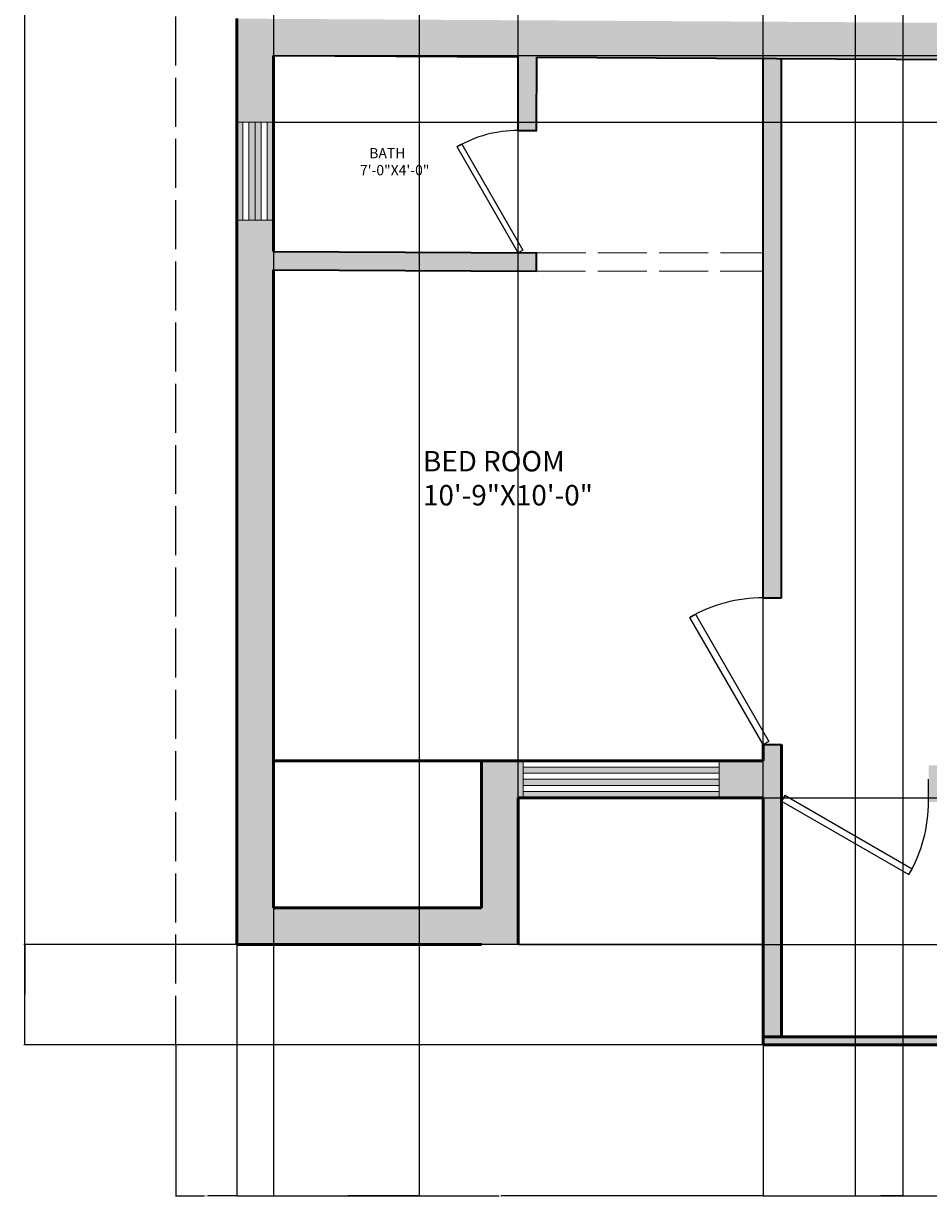
# Model space of a CAD drawing. Units: feet. Extents: x 2512 to 3087, y 1456 to 2266.
# Tile 1 of 5: x 2512 to 2734, y 1456 to 1744. Entities that reach past the tile are written whole.
import ezdxf

# ---------------------------------------------------------------- set-up
doc = ezdxf.new("R2010")
doc.units = ezdxf.units.FT
doc.linetypes.add('ACAD_ISO02W100', pattern=[15, 12, -3])
for name, color, linetype, lineweight in [('A-ANNO-DIMS', 2, 'Continuous', 18), ('A-DOOR', 240, 'Continuous', 25), ('A-GLAZ', 4, 'Continuous', 18), ('A-GLAZ-PATT', 252, 'Continuous', 13), ('A-WALL-OVHD', 8, 'ACAD_ISO02W100', 18), ('A-WALL-PATT', 252, 'Continuous', 13), ('ANNOTATION', 80, 'Continuous', 18), ('C-PROP', 8, 'ACAD_ISO02W100', 25), ('INNER WALL', 7, 'Continuous', 35), ('OPEN DOOR', 50, 'ACAD_ISO02W100', 18), ('OUTER WALL', 7, 'Continuous', 50)]:
    doc.layers.add(name, color=color, linetype=linetype, lineweight=lineweight)
doc.styles.get("Standard").update_dxf_attribs({"font": 'arial.ttf'})
doc.dimstyles.get("Standard").update_dxf_attribs({"dimtxt": 0.18, "dimasz": 0.18, "dimexe": 0.18, "dimexo": 0.0625, "dimgap": 0.09, "dimtad": 0, "dimtih": 1, "dimtoh": 1, "dimdec": 4, "dimzin": 0, "dimdsep": 46, "dimtxsty": 'Standard', "dimcen": 0.09, "dimadec": 0, "dimazin": 0, "dimtfac": 1, "dimtdec": 4, "dimtofl": 0, "dimtmove": 0, "dimatfit": 3, "dimfxl": 1, "dimtolj": 1, "dimtzin": 0, "dimarcsym": 0})

# ---------------------------------------------------------------- blocks, each defined once
blk = doc.blocks.new('*U8')
for p, q in [((0, 0), (0, 6)), ((40, 0), (40, 6))]:
    blk.add_line(p, q)
blk.add_lwpolyline([(0, 0), (34.64, -20), (35.52, -18.48), (0.87, 1.52)], close=True)
blk.add_arc((0, 0), 40, 330, 0)
blk = doc.blocks.new('*U9')
for p, q in [((-40, 0), (-40, 5)), ((0, 0), (0, 5))]:
    blk.add_line(p, q)
blk.add_lwpolyline([(0, 0), (-34.64, -20), (-35.52, -18.48), (-0.88, 1.52)], close=True)
blk.add_arc((0, 0), 40, 180, 210)
blk = doc.blocks.new('*U4')
for p, q in [((-40, 0), (-40, 6)), ((0, 0), (0, 6))]:
    blk.add_line(p, q)
blk.add_lwpolyline([(0, 0), (-34.64, -20), (-35.52, -18.48), (-0.87, 1.52)], close=True)
blk.add_arc((0, 0), 40, 180, 210)
blk = doc.blocks.new('VENT-24IN')
h = blk.add_hatch(color=256)
h.dxf.hatch_style = 1
h.paths.add_polyline_path([(24, 7.5), (24, 9), (0, 9), (0, 7.5)])
h.paths.add_polyline_path([(0, 1.5), (0, 0), (24, 0), (24, 1.5)])
h.paths.add_polyline_path([(0, 4.5), (0, 3), (24, 3), (24, 4.5)])
h.paths.add_polyline_path([(24, 4.5), (24, 6), (0, 6), (0, 4.5)])
for p, q in [((0, 9), (24, 9)), ((0, 0), (0, 9)), ((24, 9), (24, 0)), ((0, 7.5), (24, 7.5)), ((0, 6), (24, 6)), ((0, 4.5), (24, 4.5)), ((0, 3), (24, 3)), ((0, 1.5), (24, 1.5)), ((24, 0), (0, 0))]:
    blk.add_line(p, q)
blk = doc.blocks.new('*D18')
at = {"layer": 'A-ANNO-DIMS', "color": 0, "lineweight": -2, "transparency": 16777216}
for p, q in [((2549.23, 2229.02), (2512.11, 2229.02)), ((2512.29, 2228.84), (2512.29, 1861.31)), ((2512.29, 1493.41), (2512.29, 1860.94)), ((2549.23, 1493.23), (2512.11, 1493.23))]:
    blk.add_line(p, q, dxfattribs=at)
at = {"layer": 'A-ANNO-DIMS', "color": 0, "transparency": 16777216}
for points in [[(2512.26, 2228.84), (2512.32, 2228.84), (2512.29, 2229.02)], [(2512.26, 1493.41), (2512.32, 1493.41), (2512.29, 1493.23)]]:
    blk.add_solid(points, dxfattribs=at)
at = {"layer": 'Defpoints', "color": 0, "transparency": 16777216}
for p in [(2512.29, 2229.02), (2549.29, 2229.02), (2549.29, 1493.23)]:
    blk.add_point(p, dxfattribs=at)
at = {"layer": 'A-ANNO-DIMS', "color": 0, "transparency": 16777216, "insert": (2512.29, 1861.13), "char_height": 0.18, "attachment_point": 5}
blk.add_mtext('\\A1;735.8', dxfattribs=at)
blk = doc.blocks.new('*D20')
at = {"layer": 'A-ANNO-DIMS', "color": 0, "lineweight": -2, "transparency": 16777216}
for p, q in [((2564.16, 2213.23), (2512.11, 2213.23)), ((2512.29, 2213.05), (2512.29, 1853.41)), ((2512.29, 1493.41), (2512.29, 1853.05)), ((2693.16, 1493.23), (2512.11, 1493.23))]:
    blk.add_line(p, q, dxfattribs=at)
at = {"layer": 'A-ANNO-DIMS', "color": 0, "transparency": 16777216}
for points in [[(2512.26, 2213.05), (2512.32, 2213.05), (2512.29, 2213.23)], [(2512.26, 1493.41), (2512.32, 1493.41), (2512.29, 1493.23)]]:
    blk.add_solid(points, dxfattribs=at)
at = {"layer": 'Defpoints', "color": 0, "transparency": 16777216}
for p in [(2512.29, 2213.23), (2564.22, 2213.23), (2693.22, 1493.23)]:
    blk.add_point(p, dxfattribs=at)
at = {"layer": 'A-ANNO-DIMS', "color": 0, "transparency": 16777216, "insert": (2512.29, 1853.23), "char_height": 0.18, "attachment_point": 5}
blk.add_mtext('\\A1;720', dxfattribs=at)
blk = doc.blocks.new('*D21')
at = {"layer": 'A-ANNO-DIMS', "color": 0, "lineweight": -2, "transparency": 16777216}
for p, q in [((2573.22, 2204.17), (2573.22, 1456.05)), ((2608.89, 2204.17), (2608.89, 1456.05)), ((2573.4, 1456.23), (2590.66, 1456.23)), ((2608.71, 1456.23), (2591.45, 1456.23))]:
    blk.add_line(p, q, dxfattribs=at)
at = {"layer": 'A-ANNO-DIMS', "color": 0, "transparency": 16777216}
for points in [[(2573.4, 1456.26), (2573.4, 1456.2), (2573.22, 1456.23)], [(2608.71, 1456.26), (2608.71, 1456.2), (2608.89, 1456.23)]]:
    blk.add_solid(points, dxfattribs=at)
at = {"layer": 'Defpoints', "color": 0, "transparency": 16777216}
for p in [(2573.22, 2204.23), (2608.89, 2204.23), (2608.89, 1456.23)]:
    blk.add_point(p, dxfattribs=at)
at = {"layer": 'A-ANNO-DIMS', "color": 0, "transparency": 16777216, "insert": (2591.05, 1456.23), "char_height": 0.18, "attachment_point": 5}
blk.add_mtext('\\A1;35.67', dxfattribs=at)
blk = doc.blocks.new('*D22')
at = {"layer": 'A-ANNO-DIMS', "color": 0, "lineweight": -2, "transparency": 16777216}
for p, q in [((2715.72, 2204.17), (2715.72, 1456.05)), ((2727.45, 2204.17), (2727.45, 1456.05)), ((2715.9, 1456.23), (2721.13, 1456.23)), ((2727.27, 1456.23), (2722.04, 1456.23))]:
    blk.add_line(p, q, dxfattribs=at)
at = {"layer": 'A-ANNO-DIMS', "color": 0, "transparency": 16777216}
for points in [[(2715.9, 1456.26), (2715.9, 1456.2), (2715.72, 1456.23)], [(2727.27, 1456.26), (2727.27, 1456.2), (2727.45, 1456.23)]]:
    blk.add_solid(points, dxfattribs=at)
at = {"layer": 'Defpoints', "color": 0, "transparency": 16777216}
for p in [(2715.72, 2204.23), (2727.45, 2204.23), (2727.45, 1456.23)]:
    blk.add_point(p, dxfattribs=at)
at = {"layer": 'A-ANNO-DIMS', "color": 0, "transparency": 16777216, "insert": (2721.58, 1456.23), "char_height": 0.18, "attachment_point": 5}
blk.add_mtext('\\A1;11.729', dxfattribs=at)
blk = doc.blocks.new('*D25')
at = {"layer": 'A-ANNO-DIMS', "color": 0, "lineweight": -2, "transparency": 16777216}
for p, q in [((2564.22, 1517.74), (2564.22, 1456.05)), ((2549.29, 1493.17), (2549.29, 1456.05)), ((2549.47, 1456.23), (2556.37, 1456.23)), ((2564.04, 1456.23), (2557.14, 1456.23))]:
    blk.add_line(p, q, dxfattribs=at)
at = {"layer": 'A-ANNO-DIMS', "color": 0, "transparency": 16777216}
for points in [[(2549.47, 1456.26), (2549.47, 1456.2), (2549.29, 1456.23)], [(2564.04, 1456.26), (2564.04, 1456.2), (2564.22, 1456.23)]]:
    blk.add_solid(points, dxfattribs=at)
at = {"layer": 'Defpoints', "color": 0, "transparency": 16777216}
for p in [(2564.22, 1517.8), (2549.29, 1493.23), (2564.22, 1456.23)]:
    blk.add_point(p, dxfattribs=at)
at = {"layer": 'A-ANNO-DIMS', "color": 0, "transparency": 16777216, "insert": (2556.75, 1456.23), "char_height": 0.18, "attachment_point": 5}
blk.add_mtext('\\A1;14.93', dxfattribs=at)
blk = doc.blocks.new('*D26')
at = {"layer": 'A-ANNO-DIMS', "color": 0, "lineweight": -2, "transparency": 16777216}
for p, q in [((2564.22, 1517.74), (2564.22, 1456.05)), ((2693.22, 1493.17), (2693.22, 1456.05)), ((2564.4, 1456.23), (2628.44, 1456.23)), ((2693.04, 1456.23), (2629, 1456.23))]:
    blk.add_line(p, q, dxfattribs=at)
at = {"layer": 'A-ANNO-DIMS', "color": 0, "transparency": 16777216}
for points in [[(2564.4, 1456.26), (2564.4, 1456.2), (2564.22, 1456.23)], [(2693.04, 1456.26), (2693.04, 1456.2), (2693.22, 1456.23)]]:
    blk.add_solid(points, dxfattribs=at)
at = {"layer": 'Defpoints', "color": 0, "transparency": 16777216}
for p in [(2564.22, 1517.8), (2693.22, 1493.23), (2693.22, 1456.23)]:
    blk.add_point(p, dxfattribs=at)
at = {"layer": 'A-ANNO-DIMS', "color": 0, "transparency": 16777216, "insert": (2628.72, 1456.23), "char_height": 0.18, "attachment_point": 5}
blk.add_mtext('\\A1;129', dxfattribs=at)
blk = doc.blocks.new('*D27')
at = {"layer": 'A-ANNO-DIMS', "color": 0, "lineweight": -2, "transparency": 16777216}
for p, q in [((2693.22, 1493.17), (2693.22, 1456.05)), ((2828.22, 1493.17), (2828.22, 1456.05)), ((2693.4, 1456.23), (2760.44, 1456.23)), ((2828.04, 1456.23), (2761, 1456.23))]:
    blk.add_line(p, q, dxfattribs=at)
at = {"layer": 'A-ANNO-DIMS', "color": 0, "transparency": 16777216}
for points in [[(2693.4, 1456.26), (2693.4, 1456.2), (2693.22, 1456.23)], [(2828.04, 1456.26), (2828.04, 1456.2), (2828.22, 1456.23)]]:
    blk.add_solid(points, dxfattribs=at)
at = {"layer": 'Defpoints', "color": 0, "transparency": 16777216}
for p in [(2693.22, 1493.23), (2828.22, 1493.23), (2828.22, 1456.23)]:
    blk.add_point(p, dxfattribs=at)
at = {"layer": 'A-ANNO-DIMS', "color": 0, "transparency": 16777216, "insert": (2760.72, 1456.23), "char_height": 0.18, "attachment_point": 5}
blk.add_mtext('\\A1;135', dxfattribs=at)
blk = doc.blocks.new('*D29')
at = {"layer": 'A-ANNO-DIMS', "color": 0, "lineweight": -2, "transparency": 16777216}
for p, q in [((2633.22, 1517.86), (2633.22, 2266.2)), ((2633.4, 2266.02), (2663, 2266.02)), ((2693.04, 2266.02), (2663.44, 2266.02)), ((2693.22, 1517.86), (2693.22, 2266.2))]:
    blk.add_line(p, q, dxfattribs=at)
at = {"layer": 'A-ANNO-DIMS', "color": 0, "transparency": 16777216}
for points in [[(2633.4, 2266.05), (2633.4, 2265.99), (2633.22, 2266.02)], [(2693.04, 2266.05), (2693.04, 2265.99), (2693.22, 2266.02)]]:
    blk.add_solid(points, dxfattribs=at)
at = {"layer": 'Defpoints', "color": 0, "transparency": 16777216}
for p in [(2693.22, 2266.02), (2633.22, 1517.8), (2693.22, 1517.8)]:
    blk.add_point(p, dxfattribs=at)
at = {"layer": 'A-ANNO-DIMS', "color": 0, "transparency": 16777216, "insert": (2663.22, 2266.02), "char_height": 0.18, "attachment_point": 5}
blk.add_mtext('\\A1;60', dxfattribs=at)
blk = doc.blocks.new('*D30')
at = {"layer": 'A-ANNO-DIMS', "color": 0, "lineweight": -2, "transparency": 16777216}
for p, q in [((2633.28, 1553.8), (3087.03, 1553.8)), ((3086.85, 1553.62), (3086.85, 1535.98)), ((3086.85, 1517.98), (3086.85, 1535.62)), ((2633.28, 1517.8), (3087.03, 1517.8))]:
    blk.add_line(p, q, dxfattribs=at)
at = {"layer": 'A-ANNO-DIMS', "color": 0, "transparency": 16777216}
for points in [[(3086.82, 1553.62), (3086.88, 1553.62), (3086.85, 1553.8)], [(3086.82, 1517.98), (3086.88, 1517.98), (3086.85, 1517.8)]]:
    blk.add_solid(points, dxfattribs=at)
at = {"layer": 'Defpoints', "color": 0, "transparency": 16777216}
for p in [(2633.22, 1553.8), (3086.85, 1553.8), (2633.22, 1517.8)]:
    blk.add_point(p, dxfattribs=at)
at = {"layer": 'A-ANNO-DIMS', "color": 0, "transparency": 16777216, "insert": (3086.85, 1535.8), "char_height": 0.18, "attachment_point": 5}
blk.add_mtext('\\A1;36', dxfattribs=at)
blk = doc.blocks.new('*D31')
at = {"layer": 'A-ANNO-DIMS', "color": 0, "lineweight": -2, "transparency": 16777216}
for p, q in [((2693.16, 1517.8), (2512.11, 1517.8)), ((2512.29, 1517.62), (2512.29, 1505.7)), ((2512.29, 1493.41), (2512.29, 1505.33)), ((2693.16, 1493.23), (2512.11, 1493.23))]:
    blk.add_line(p, q, dxfattribs=at)
at = {"layer": 'A-ANNO-DIMS', "color": 0, "transparency": 16777216}
for points in [[(2512.26, 1517.62), (2512.32, 1517.62), (2512.29, 1517.8)], [(2512.26, 1493.41), (2512.32, 1493.41), (2512.29, 1493.23)]]:
    blk.add_solid(points, dxfattribs=at)
at = {"layer": 'Defpoints', "color": 0, "transparency": 16777216}
for p in [(2512.29, 1517.8), (2693.22, 1517.8), (2693.22, 1493.23)]:
    blk.add_point(p, dxfattribs=at)
at = {"layer": 'A-ANNO-DIMS', "color": 0, "transparency": 16777216, "insert": (2512.29, 1505.52), "char_height": 0.18, "attachment_point": 5}
blk.add_mtext('\\A1;24.57', dxfattribs=at)
blk = doc.blocks.new('*D49')
at = {"layer": 'A-ANNO-DIMS', "color": 0, "lineweight": -2, "transparency": 16777216}
for p, q in [((2573.28, 1735.68), (3087.03, 1735.68)), ((3086.85, 1735.5), (3086.85, 1727.7)), ((3086.85, 1719.55), (3086.85, 1727.34)), ((2573.28, 1719.37), (3087.03, 1719.37))]:
    blk.add_line(p, q, dxfattribs=at)
at = {"layer": 'A-ANNO-DIMS', "color": 0, "transparency": 16777216}
for points in [[(3086.82, 1735.5), (3086.88, 1735.5), (3086.85, 1735.68)], [(3086.82, 1719.55), (3086.88, 1719.55), (3086.85, 1719.37)]]:
    blk.add_solid(points, dxfattribs=at)
at = {"layer": 'Defpoints', "color": 0, "transparency": 16777216}
for p in [(2573.22, 1735.68), (3086.85, 1735.68), (2573.22, 1719.37)]:
    blk.add_point(p, dxfattribs=at)
at = {"layer": 'A-ANNO-DIMS', "color": 0, "transparency": 16777216, "insert": (3086.85, 1727.52), "char_height": 0.18, "attachment_point": 5}
blk.add_mtext('\\A1;16.305', dxfattribs=at)

msp = doc.modelspace()

# ---------------------------------------------------------------- hatches: boundary and pattern name
at = {"layer": 'A-GLAZ-PATT'}
h = msp.add_hatch(color=256, dxfattribs=at)
h.dxf.hatch_style = 1
h.paths.add_polyline_path([(2634.4194, 1561.3011), (2634.4194, 1559.8011), (2682.4194, 1559.8011), (2682.4194, 1561.3011)])
h.paths.add_polyline_path([(2682.4194, 1556.8011), (2682.4194, 1558.3011), (2634.4194, 1558.3011), (2634.4194, 1556.8011)])
h.paths.add_polyline_path([(2682.4194, 1553.8011), (2682.4194, 1555.3011), (2634.4194, 1555.3011), (2634.4194, 1553.8011)])
at = {"layer": 'A-WALL-PATT'}
h = msp.add_hatch(color=256, dxfattribs=at)
h.dxf.hatch_style = 1
h.paths.add_polyline_path([(3035.2185, 1915.2872), (3026.2185, 1915.2872), (3026.2185, 1912.7316), (2936.2185, 1912.7316), (2936.2185, 2001.7316), (2931.7185, 2001.7316), (2931.7185, 1912.7316), (2808.7185, 1912.7316), (2808.7185, 1903.7316), (3026.2185, 1903.7316), (3026.2185, 1816.7316), (2808.7185, 1816.7316), (2808.7185, 1807.7316), (2823.7185, 1807.7316), (2823.7185, 1638.2316), (2828.2185, 1638.2316), (2828.2185, 1674.2316), (2828.2185, 1678.7316), (2828.2185, 1807.7316), (3026.2185, 1807.7316), (3026.2185, 1735.7316), (3002.2185, 1735.7316), (3002.2546, 1726.7316), (3011.2546, 1726.7316), (3035.2185, 1726.7316)])
h.paths.add_polyline_path([(3035.2185, 2001.7316), (2990.2185, 2001.7316), (2972.2185, 2001.7316), (2972.2185, 1996.7316), (3026.2185, 1996.7316), (3026.2185, 1963.2872), (3035.2185, 1963.2872)], flags=17)
h.paths.add_polyline_path([(3041.2185, 2010.7316), (2990.2185, 2010.7316), (2990.2185, 2001.7316), (3035.2185, 2001.7316), (3041.2185, 2001.7316)])
h.paths.add_polyline_path([(3044.2185, 2085.7316), (3044.2185, 2088.2316), (3041.2185, 2088.2316), (3041.2185, 2006.2316), (3044.2185, 2006.2316)])
h.paths.add_polyline_path([(3041.2185, 2090.2316), (2975.2185, 2090.2316), (2975.2185, 2090.2254), (2966.2185, 2090.2254), (2825.2185, 2090.2316), (2825.2185, 2091.7316), (2820.7185, 2091.7316), (2820.7185, 2085.7316), (2820.7185, 2084.2316), (2825.2185, 2084.2316), (2825.2185, 2085.7316), (2990.2185, 2085.7316), (2990.2185, 2046.7316), (2999.2185, 2046.7316), (2999.2185, 2085.7316), (3041.2185, 2085.7316)])
h.paths.add_polyline_path([(3035.2185, 2213.2316), (2918.3922, 2213.2316), (2918.3922, 2204.2316), (3026.2185, 2204.2316), (3026.2185, 2144.2316), (2966.2185, 2144.2316), (2966.2185, 2135.213), (2975.2185, 2135.213), (2975.2185, 2135.2316), (3035.2185, 2135.2316)])
h.paths.add_polyline_path([(2870.3922, 2213.2316), (2809.1404, 2213.2316), (2809.1404, 2204.2316), (2820.7185, 2204.2316), (2820.7185, 2162.2316), (2825.2185, 2162.2316), (2825.2185, 2204.2316), (2870.3922, 2204.2316)])
h.paths.add_polyline_path([(2785.1404, 2213.2316), (2751.447, 2213.2316), (2751.447, 2204.2316), (2763.7185, 2204.2316), (2763.7185, 2127.7316), (2825.2185, 2127.7316), (2825.2185, 2132.2316), (2820.7185, 2132.2316), (2772.7185, 2132.2316), (2772.7185, 2204.2316), (2785.1404, 2204.2316)])
h.paths.add_polyline_path([(2727.447, 2213.2316), (2656.8898, 2213.2316), (2656.8898, 2204.2316), (2711.2185, 2204.2316), (2711.2185, 2124.7316), (2715.7185, 2124.7316), (2715.7185, 2127.7316), (2733.7185, 2127.7316), (2733.7185, 2132.2316), (2715.7185, 2132.2316), (2715.7185, 2204.2316), (2727.447, 2204.2316)], flags=17)
h.paths.add_polyline_path([(2608.8898, 2213.2316), (2564.2185, 2213.2316), (2564.2185, 2079.7316), (2609.2185, 2079.7316), (2609.2185, 2037.7316), (2618.2185, 2037.7316), (2618.2185, 2079.7316), (2763.7185, 2079.7316), (2763.7185, 2007.7316), (2654.2185, 2007.7316), (2654.2185, 2003.2316), (2763.7185, 2003.2316), (2763.7185, 1891.0755), (2772.7185, 1891.0234), (2772.7185, 1903.7316), (2772.7185, 2088.7316), (2573.2185, 2088.7316), (2573.2185, 2204.2316), (2608.8898, 2204.2316)])
h.paths.add_polyline_path([(2567.2185, 2079.7316), (2564.2185, 2079.7316), (2564.2185, 2007.7316), (2567.2185, 2007.7316)], flags=17)
h.paths.add_polyline_path([(2618.2185, 2007.7316), (2564.2185, 2007.7316), (2564.2185, 2003.2171), (2573.2185, 2003.2171), (2573.2185, 2003.2316), (2618.2185, 2003.2316)], flags=17)
h.paths.add_polyline_path([(2573.2185, 1955.2171), (2564.2185, 1955.2171), (2564.2185, 1904.096), (2573.2185, 1904.096)], flags=17)
h.paths.add_polyline_path([(2573.2185, 1851.677), (2603.2185, 1851.5035), (2603.2195, 1856.0035), (2573.2185, 1856.1771), (2573.2185, 1856.096), (2564.2185, 1856.096), (2564.2185, 1785.728), (2594.2185, 1785.5544), (2600.2185, 1785.5197), (2637.7185, 1785.3028), (2637.7185, 1855.8039), (2633.2185, 1855.83), (2633.2185, 1789.8289), (2573.2185, 1790.176)])
h.paths.add_polyline_path([(2772.7185, 1855.0228), (2767.3185, 1855.0228), (2767.3004, 1855.0542), (2673.7185, 1855.5956), (2673.7185, 1851.0956), (2763.7185, 1850.575), (2763.7185, 1743.5732), (2564.2185, 1744.7273), (2564.2185, 1719.3701), (2573.2185, 1719.3701), (2573.2185, 1735.6751), (2633.2185, 1735.328), (2633.2185, 1717.3272), (2637.7185, 1717.3272), (2637.7185, 1735.302), (2772.7185, 1734.521)])
h.paths.add_polyline_path([(2697.7185, 1734.9549), (2693.2185, 1734.9809), (2693.2185, 1602.8011), (2697.7185, 1602.8011)])
h.paths.add_polyline_path([(2823.7185, 1561.2231), (2733.7185, 1561.7437), (2733.7185, 1552.7436), (2823.7185, 1552.2229)])
h.paths.add_polyline_path([(2697.7185, 1566.8011), (2693.2185, 1566.8011), (2693.2185, 1562.8011), (2682.4194, 1562.8011), (2682.4194, 1553.8011), (2693.2185, 1553.8011), (2693.2185, 1495.2316), (2697.7185, 1495.2316)])
h.paths.add_polyline_path([(2828.2185, 1495.2316), (2693.2185, 1495.2316), (2693.2185, 1493.2316), (2828.2185, 1493.2316)])
h.paths.add_polyline_path([(2828.2185, 1602.2316), (2823.7185, 1602.2316), (2823.7185, 1495.2316), (2828.2185, 1495.2316)])
h.paths.add_polyline_path([(3035.2185, 1523.0765), (3026.2185, 1523.0765), (3026.2185, 1513.7316), (2828.2185, 1513.7316), (2828.2185, 1504.7316), (3035.2185, 1504.7316)])
h.paths.add_polyline_path([(3026.2185, 1602.2316), (2906.2185, 1602.2316), (2906.2185, 1644.2316), (2901.7185, 1644.2316), (2901.7185, 1597.7316), (3026.2185, 1597.7316)])
h.paths.add_polyline_path([(3035.2185, 1678.7316), (2864.2185, 1678.7316), (2864.2185, 1674.2316), (3026.2185, 1674.2316), (3026.2185, 1642.5123), (3035.2185, 1642.5123)], flags=17)
h.paths.add_polyline_path([(3035.2185, 1618.5123), (3026.2185, 1618.5123), (3026.2185, 1571.0765), (3035.2185, 1571.0765)])
h = msp.add_hatch(color=256, dxfattribs=at)
h.dxf.hatch_style = 1
h.paths.add_polyline_path([(2573.2185, 1683.1742), (2637.6925, 1682.8012), (2637.6947, 1687.3013), (2573.2185, 1687.6743), (2573.2185, 1695.3702), (2564.2185, 1695.3702), (2564.2185, 1517.8011), (2624.2185, 1517.8011), (2633.2185, 1517.8011), (2633.2185, 1553.8011), (2634.4194, 1553.8011), (2634.4194, 1562.8011), (2624.2185, 1562.8011), (2624.2185, 1526.8011), (2573.2185, 1526.8011)])
h.paths.add_polyline_path([(2573.2185, 1735.6751), (2633.2185, 1735.328), (2633.2185, 1717.3272), (2637.7096, 1717.3272), (2637.7185, 1735.302), (2772.7185, 1734.521), (2772.7185, 1855.0228), (2673.7185, 1855.5956), (2673.7185, 1851.0956), (2763.7185, 1850.575), (2763.7185, 1743.5732), (2564.2185, 1744.7273), (2564.2185, 1719.3701), (2573.2185, 1719.3701)])
h.paths.add_polyline_path([(2828.2185, 1807.7316), (3026.2185, 1807.7316), (3026.2185, 1735.7316), (3002.2185, 1735.7316), (3002.2546, 1726.7316), (3011.2546, 1726.7316), (3035.2185, 1726.7316), (3035.2185, 1915.2872), (3026.2185, 1915.2872), (3026.2185, 1912.7316), (2936.2185, 1912.7316), (2936.2185, 2001.7316), (2931.7185, 2001.7316), (2931.7185, 1912.7316), (2808.7185, 1912.7316), (2808.7185, 1903.7316), (3026.2185, 1903.7316), (3026.2185, 1816.7316), (2808.7185, 1816.7316), (2808.7185, 1807.7316), (2823.7185, 1807.7316), (2823.7185, 1638.2316), (2828.2185, 1638.2316), (2828.2185, 1674.2316), (2828.2185, 1678.7316)])
h.paths.add_polyline_path([(3035.2185, 1678.7316), (2864.2185, 1678.7316), (2864.2185, 1674.2316), (3026.2185, 1674.2316), (3026.2185, 1642.5123), (3035.2185, 1642.5123)], flags=17)
h.paths.add_polyline_path([(3035.2185, 1618.5123), (3026.2185, 1618.5123), (3026.2185, 1571.0765), (3035.2185, 1571.0765)])
h.paths.add_polyline_path([(3026.2185, 1602.2316), (2906.2185, 1602.2316), (2906.2185, 1644.2316), (2901.7185, 1644.2316), (2901.7185, 1597.7316), (3026.2185, 1597.7316)])
h.paths.add_polyline_path([(3035.2185, 1523.0765), (3026.2185, 1523.0765), (3026.2185, 1513.7316), (2828.2185, 1513.7316), (2828.2185, 1504.7316), (3035.2185, 1504.7316)])
h.paths.add_polyline_path([(2828.2185, 1495.2316), (2693.2185, 1495.2316), (2693.2185, 1493.2316), (2828.2185, 1493.2316)])
h.paths.add_polyline_path([(2828.2185, 1602.2316), (2823.7185, 1602.2316), (2823.7185, 1495.2316), (2828.2185, 1495.2316)])
h.paths.add_polyline_path([(2823.7185, 1561.2231), (2733.7185, 1561.7437), (2733.7185, 1552.7436), (2823.7185, 1552.2229)])
h.paths.add_polyline_path([(2697.7185, 1566.8011), (2693.2185, 1566.8011), (2693.2185, 1562.8011), (2682.4194, 1562.8011), (2682.4194, 1553.8011), (2693.2185, 1553.8011), (2693.2185, 1495.2316), (2697.7185, 1495.2316)])
h.paths.add_polyline_path([(2697.7185, 1734.9549), (2693.2185, 1734.9809), (2693.2185, 1602.8011), (2697.7185, 1602.8011)])
h.paths.add_polyline_path([(2573.2185, 1851.677), (2603.2185, 1851.5035), (2603.2195, 1856.0035), (2573.2185, 1856.1771), (2573.2185, 1856.096), (2564.2185, 1856.096), (2564.2185, 1785.728), (2594.2185, 1785.5544), (2600.2185, 1785.5197), (2637.7185, 1785.3028), (2637.7185, 1855.8039), (2633.2185, 1855.83), (2633.2185, 1789.8289), (2573.2185, 1790.176)])
h.paths.add_polyline_path([(2573.2185, 1955.2171), (2564.2185, 1955.2171), (2564.2185, 1904.096), (2573.2185, 1904.096)])
h.paths.add_polyline_path([(2618.2185, 2007.7316), (2564.2185, 2007.7316), (2564.2185, 2003.2171), (2573.2185, 2003.2171), (2573.2185, 2003.2316), (2618.2185, 2003.2316)])
h.paths.add_polyline_path([(2567.2185, 2079.7316), (2564.2185, 2079.7316), (2564.2185, 2007.7316), (2567.2185, 2007.7316)])

# ---------------------------------------------------------------- linework, layer by layer
at = {"layer": 'A-GLAZ'}
for p, q in [((2634.4194, 1562.8011), (2682.4194, 1562.8011)), ((2634.4194, 1553.8011), (2634.4194, 1562.8011)), ((2634.4194, 1561.3011), (2682.4194, 1561.3011)), ((2682.4194, 1562.8011), (2682.4194, 1553.8011)), ((2634.4194, 1559.8011), (2682.4194, 1559.8011)), ((2634.4194, 1558.3011), (2682.4194, 1558.3011)), ((2634.4194, 1558.3011), (2682.4194, 1558.3011)), ((2634.4194, 1556.8011), (2682.4194, 1556.8011)), ((2634.4194, 1555.3011), (2682.4194, 1555.3011)), ((2682.4194, 1553.8011), (2634.4194, 1553.8011))]:
    msp.add_line(p, q, dxfattribs=at)
at = {"layer": 'A-WALL-OVHD'}
msp.add_line((2624.2185, 1517.8011), (2693.2185, 1517.8011), dxfattribs=at)
at = {"layer": 'C-PROP'}
for p, q in [((2549.289, 1493.2316), (2549.289, 2229.0217)), ((2693.2185, 1493.2316), (2549.289, 1493.2316))]:
    msp.add_line(p, q, dxfattribs=at)
at = {"layer": 'INNER WALL'}
for p, q in [((2573.2185, 1735.6751), (2633.2185, 1735.328)), ((2633.2185, 1717.3272), (2633.2185, 1735.328)), ((2637.7096, 1717.3272), (2637.7185, 1735.302)), ((2637.7185, 1735.302), (2772.7185, 1734.521)), ((2693.2185, 1602.8011), (2693.2185, 1734.9809)), ((2697.7185, 1602.8011), (2697.7185, 1734.9549)), ((2633.2185, 1717.3272), (2637.7185, 1717.3272)), ((2573.2185, 1687.6743), (2637.7185, 1687.3012)), ((2637.6925, 1682.8012), (2637.6947, 1687.3272)), ((2573.2185, 1683.1742), (2637.6925, 1682.8012)), ((2693.2185, 1602.8011), (2693.2185, 1683.1742)), ((2693.2185, 1602.8011), (2697.7185, 1602.8011)), ((2693.2185, 1566.8011), (2697.7185, 1566.8011))]:
    msp.add_line(p, q, dxfattribs=at)
at = {"layer": 'OPEN DOOR'}
for p, q in [((2637.7185, 1687.3012), (2693.2185, 1687.3012)), ((2637.6925, 1682.8012), (2693.2185, 1682.8012))]:
    msp.add_line(p, q, dxfattribs=at)
at = {"layer": 'OUTER WALL'}
for p, q in [((2564.2185, 1517.8011), (2564.2185, 1744.7273)), ((2573.2185, 1687.6743), (2573.2185, 1735.6751)), ((2573.2185, 1526.8011), (2573.2185, 1683.1742)), ((2693.2185, 1562.8011), (2693.2185, 1566.8011)), ((2693.2185, 1562.8011), (2693.2185, 1566.8011)), ((2697.7185, 1495.2316), (2697.7185, 1566.8011)), ((2624.2185, 1562.8011), (2573.2185, 1562.8011)), ((2624.2185, 1562.8011), (2693.2185, 1562.8011)), ((2624.2185, 1562.8011), (2624.2185, 1526.8011)), ((2633.2185, 1553.8011), (2693.2185, 1553.8011)), ((2633.2185, 1553.8011), (2633.2185, 1517.8011)), ((2693.2185, 1493.2316), (2693.2185, 1553.8011)), ((2693.2185, 1502.2316), (2693.2185, 1553.8011)), ((2697.6664, 1552.9521), (2697.7185, 1552.9518)), ((2624.2185, 1526.8011), (2573.2185, 1526.8011)), ((2624.2185, 1517.8011), (2564.2185, 1517.8011)), ((2828.2185, 1495.2316), (2693.2185, 1495.2316)), ((2693.2185, 1493.2316), (2828.2185, 1493.2316))]:
    msp.add_line(p, q, dxfattribs=at)

# ---------------------------------------------------------------- block references
at = {"layer": 'A-DOOR', "rotation": 270}
for name, p, xscale, yscale, zscale in [('*U4', (2633.2185, 1687.3272), 0.7500000000000038, 0.7500000000000038, 0.7500000000000038), ('*U9', (2693.2185, 1566.8011), 0.899999999999959, 0.899999999999959, 0.899999999999959)]:
    msp.add_blockref(name, p, dxfattribs=dict(at, xscale=xscale, yscale=yscale, zscale=zscale))
at = {"layer": 'A-DOOR', "xscale": 0.899999999999959, "yscale": 0.899999999999959, "zscale": 0.899999999999959}
msp.add_blockref('*U8', (2697.7185, 1552.9518), dxfattribs=at)
at = {"layer": 'A-GLAZ', "rotation": 269.9999999999984}
msp.add_blockref('VENT-24IN', (2564.2189, 1719.3702), dxfattribs=at)

# ---------------------------------------------------------------- texts
at = {"layer": 'ANNOTATION', "attachment_point": 1}
for s, width, insert, char_height in [('   BATH\\P7\'-0"X4\'-0"', 16.842597, (2594.4173, 1713.0101), 2.5), ('\\A1;BED ROOM\\P10\'-9"X10\'-0"', 38.558323, (2609.8693, 1638.7681), 5)]:
    msp.add_mtext_dynamic_manual_height_columns(s, width=width, gutter_width=12.5, heights=[0], dxfattribs=dict(at, insert=insert, char_height=char_height))

# ---------------------------------------------------------------- dimensions: what is measured, and where the dimension line sits
at = {"layer": 'A-ANNO-DIMS'}
for base, p1, p2, override, picture, middle in [((2693.2185, 2266.0217), (2633.2185, 1517.8011), (2693.2185, 1517.8011), {"dimdec": 0, "dimlfac": 1, "dimrnd": 0, "dimzin": 0, "dimdsep": 46, "dimlunit": 2}, '*D29', (2663.2185, 2266.0217)), ((2608.8898, 1456.2316), (2573.2185, 2204.2316), (2608.8898, 2204.2316), {"dimdec": 2, "dimlfac": 1, "dimrnd": 0, "dimzin": 0, "dimdsep": 46, "dimlunit": 2}, '*D21', (2591.0541, 1456.2316)), ((2727.44702, 1456.23162), (2715.71848, 2204.23162), (2727.44702, 2204.23162), {"dimdec": 3, "dimlfac": 1, "dimrnd": 0, "dimzin": 0, "dimdsep": 46, "dimlunit": 2}, '*D22', (2721.58275, 1456.23162)), ((2564.2185, 1456.2316), (2549.289, 1493.2316), (2564.2185, 1517.8011), {"dimdec": 2, "dimlfac": 1, "dimrnd": 0, "dimzin": 0, "dimdsep": 46, "dimlunit": 2}, '*D25', (2556.7537, 1456.2316)), ((2693.2185, 1456.2316), (2564.2185, 1517.8011), (2693.2185, 1493.2316), {"dimdec": 0, "dimlfac": 1, "dimrnd": 0, "dimzin": 0, "dimdsep": 46, "dimlunit": 2}, '*D26', (2628.7185, 1456.2316)), ((2828.2185, 1456.2316), (2693.2185, 1493.2316), (2828.2185, 1493.2316), {"dimdec": 0, "dimlfac": 1, "dimrnd": 0, "dimzin": 0, "dimdsep": 46, "dimlunit": 2}, '*D27', (2760.7185, 1456.2316))]:
    dim = msp.add_linear_dim(base=base, p1=p1, p2=p2, dimstyle='Standard', override=override, dxfattribs=at)
    dim.commit()
    dim.dimension.update_dxf_attribs({"geometry": picture, "text_midpoint": middle})
for base, p1, p2, override, picture, middle in [((2512.289, 2229.0217), (2549.289, 1493.2316), (2549.289, 2229.0217), {"dimdec": 1, "dimlfac": 1, "dimrnd": 0, "dimzin": 0, "dimdsep": 46, "dimlunit": 2}, '*D18', (2512.289, 1861.1267)), ((2512.289, 2213.2316), (2693.2185, 1493.2316), (2564.2185, 2213.2316), {"dimdec": 0, "dimlfac": 1, "dimrnd": 0, "dimzin": 0, "dimdsep": 46, "dimlunit": 2}, '*D20', (2512.289, 1853.2316)), ((3086.8469, 1735.6751), (2573.2185, 1719.3701), (2573.2185, 1735.6751), {"dimdec": 3, "dimlfac": 1, "dimrnd": 0, "dimzin": 0, "dimdsep": 46, "dimlunit": 2}, '*D49', (3086.8469, 1727.5226)), ((3086.8469, 1553.8011), (2633.2185, 1517.8011), (2633.2185, 1553.8011), {"dimdec": 0, "dimlfac": 1, "dimrnd": 0, "dimzin": 0, "dimdsep": 46, "dimlunit": 2}, '*D30', (3086.8469, 1535.8011)), ((2512.289, 1517.8011), (2693.2185, 1493.2316), (2693.2185, 1517.8011), {"dimdec": 2, "dimlfac": 1, "dimrnd": 0, "dimzin": 0, "dimdsep": 46, "dimlunit": 2}, '*D31', (2512.289, 1505.5164))]:
    dim = msp.add_linear_dim(base=base, p1=p1, p2=p2, angle=90, dimstyle='Standard', override=override, dxfattribs=at)
    dim.commit()
    dim.dimension.update_dxf_attribs({"geometry": picture, "text_midpoint": middle})

doc.saveas('drawing.dxf')
